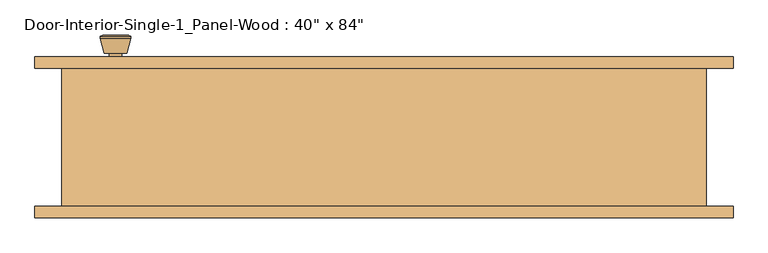
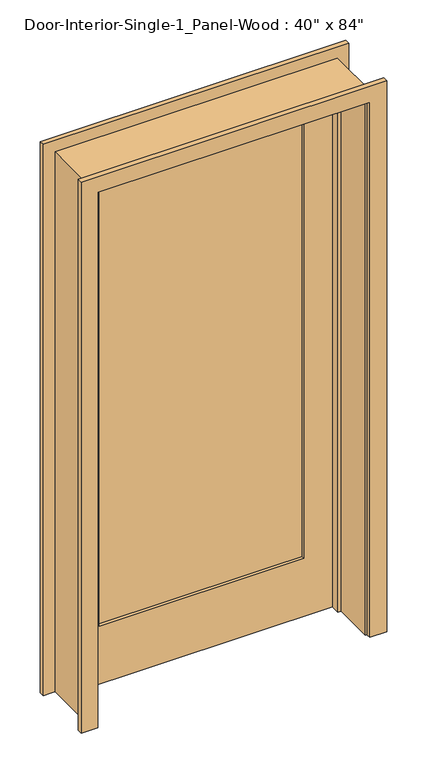
"""IFC4 building model written with IfcOpenShell, lengths in millimetres: door geometry."""

from ifc_helpers import new_model, si_unit, point, frame, frame_2d, origin, place, context, project, spatial, polyline, circle_curve, trimmed, segment, composite_curve, outline, extrude, faceted_brep, source, transform, mapped, element, save
from ifc_brep_helpers import plane_surface, cylinder_surface, revolved_surface, advanced_brep


def door_3a9a63a9(model_context):
    return source(origin(), model_context, "Body", "SolidModel", [
        advanced_brep(
        [(-444.5, 70.2, 914.4), (-434.5, 70.2, 914.4), (-454.5, 70.2, 914.4), (-424.0241324, 21.2, 914.4), (-444.5, 21.2, 914.4), (-464.9758676, 21.2, 914.4), (-419.5, 23.0278681, 914.4), (-469.5, 23.0278681, 914.4), (-419.5, 26.4915463, 914.4), (-469.5, 26.4915463, 914.4), (-425.863764, 51.2, 914.4), (-463.136236, 51.2, 914.4), (-434.5, 51.2, 914.4), (-454.5, 51.2, 914.4)],
        [
            (0, 1),
            (1, 2, circle_curve(frame((-444.5, 70.2, 914.4), z_axis=(0.0, 1.0, 0.0), x_axis=(-1.0, 0.0, 0.0)), 10.0)),
            (2, 0),
            (2, 1, circle_curve(frame((-444.5, 70.2, 914.4), z_axis=(0.0, 1.0, 0.0), x_axis=(-1.0, 0.0, 0.0)), 10.0)),
            (3, 4),
            (4, 5),
            (5, 3, circle_curve(frame((-444.5, 21.2, 914.4), z_axis=(0.0, -1.0, 0.0), x_axis=(-1.0, 0.0, 0.0)), 20.4758676)),
            (3, 5, circle_curve(frame((-444.5, 21.2, 914.4), z_axis=(0.0, -1.0, 0.0), x_axis=(-1.0, 0.0, 0.0)), 20.4758676)),
            (6, 3),
            (5, 7),
            (7, 6, circle_curve(frame((-444.5, 23.0278681, 914.4), z_axis=(0.0, -1.0, 0.0), x_axis=(-1.0, 0.0, 0.0)), 25.0)),
            (6, 7, circle_curve(frame((-444.5, 23.0278681, 914.4), z_axis=(0.0, -1.0, 0.0), x_axis=(-1.0, 0.0, 0.0)), 25.0)),
            (8, 6),
            (7, 9),
            (9, 8, circle_curve(frame((-444.5, 26.4915463, 914.4), z_axis=(0.0, -1.0, 0.0), x_axis=(-1.0, 0.0, 0.0)), 25.0)),
            (8, 9, circle_curve(frame((-444.5, 26.4915463, 914.4), z_axis=(0.0, -1.0, 0.0), x_axis=(-1.0, 0.0, 0.0)), 25.0)),
            (10, 8),
            (9, 11),
            (11, 10, circle_curve(frame((-444.5, 51.2, 914.4), z_axis=(0.0, -1.0, 0.0), x_axis=(-1.0, 0.0, 0.0)), 18.636236)),
            (10, 11, circle_curve(frame((-444.5, 51.2, 914.4), z_axis=(0.0, -1.0, 0.0), x_axis=(-1.0, 0.0, 0.0)), 18.636236)),
            (12, 10),
            (11, 13),
            (13, 12, circle_curve(frame((-444.5, 51.2, 914.4), z_axis=(0.0, -1.0, 0.0), x_axis=(-1.0, 0.0, 0.0)), 10.0)),
            (12, 13, circle_curve(frame((-444.5, 51.2, 914.4), z_axis=(0.0, -1.0, 0.0), x_axis=(-1.0, 0.0, 0.0)), 10.0)),
            (1, 12),
            (13, 2),
        ],
        [
            plane_surface(frame((-444.5, 70.2, 914.4), z_axis=(0.0, 1.0, 0.0), x_axis=(-1.0, 0.0, 0.0))),
            plane_surface(frame((-444.5, 21.2, 914.4), z_axis=(0.0, -1.0, 0.0), x_axis=(-1.0, 0.0, 0.0))),
            revolved_surface(polyline([(-464.9758676, 21.2, 914.4), (-469.5, 23.0278681, 914.4)]), (-444.5, 70.2, 914.4), (0.0, 1.0, 0.0)),
            cylinder_surface(frame((-444.5, 70.2, 914.4), z_axis=(0.0, 1.0, 0.0), x_axis=(-1.0, 0.0, 0.0)), 25.0),
            revolved_surface(polyline([(-469.5, 26.4915463, 914.4), (-463.136236, 51.2, 914.4)]), (-444.5, 70.2, 914.4), (0.0, 1.0, 0.0)),
            plane_surface(frame((-444.5, 51.2, 914.4), z_axis=(0.0, 1.0, 0.0), x_axis=(-1.0, 0.0, 0.0))),
            cylinder_surface(frame((-444.5, 70.2, 914.4), z_axis=(0.0, 1.0, 0.0), x_axis=(-1.0, 0.0, 0.0)), 10.0),
        ],
        [
            (0, [[1, 2, 3]]),
            (0, [[-3, 4, -1]]),
            (1, [[5, 6, 7]]),
            (1, [[-6, -5, 8]]),
            (2, [[9, -7, 10, 11]]),
            (2, [[-10, -8, -9, 12]]),
            (3, [[13, -11, 14, 15]]),
            (3, [[-14, -12, -13, 16]]),
            (4, [[17, -15, 18, 19]]),
            (4, [[-18, -16, -17, 20]]),
            (5, [[21, -19, 22, 23]]),
            (5, [[-22, -20, -21, 24]]),
            (6, [[25, -23, 26, -2]]),
            (6, [[-26, -24, -25, -4]]),
        ],
    ),
        extrude(outline(composite_curve([segment(trimmed(circle_curve(frame_2d((914.4, -444.5)), 30.0), [point((914.4, -474.5))], [point((914.4, -414.5))], False, "CARTESIAN"), True, "CONTINUOUS"), segment(trimmed(circle_curve(frame_2d((914.4, -444.5)), 30.0), [point((914.4, -414.5))], [point((914.4, -474.5))], False, "CARTESIAN"), True, "CONTINUOUS")], self_intersect=False)), frame((0.0, 70.2, 0.0), z_axis=(0.0, 1.0, 0.0), x_axis=(0.0, 0.0, 1.0)), (0.0, 0.0, 1.0), 6.0),
        advanced_brep(
        [(-444.5, 117.125, 914.4), (-454.5, 117.125, 914.4), (-434.5, 117.125, 914.4), (-424.0241324, 166.125, 914.4), (-464.9758676, 166.125, 914.4), (-444.5, 166.125, 914.4), (-419.5, 164.2971319, 914.4), (-469.5, 164.2971319, 914.4), (-419.5, 160.8334537, 914.4), (-469.5, 160.8334537, 914.4), (-425.863764, 136.125, 914.4), (-463.136236, 136.125, 914.4), (-434.5, 136.125, 914.4), (-454.5, 136.125, 914.4)],
        [
            (0, 1),
            (1, 2, circle_curve(frame((-444.5, 117.125, 914.4), z_axis=(0.0, -1.0, 0.0), x_axis=(-1.0, 0.0, 0.0)), 10.0)),
            (2, 0),
            (2, 1, circle_curve(frame((-444.5, 117.125, 914.4), z_axis=(0.0, -1.0, 0.0), x_axis=(-1.0, 0.0, 0.0)), 10.0)),
            (3, 4, circle_curve(frame((-444.5, 166.125, 914.4), z_axis=(0.0, 1.0, 0.0), x_axis=(-1.0, 0.0, 0.0)), 20.4758676)),
            (4, 5),
            (5, 3),
            (4, 3, circle_curve(frame((-444.5, 166.125, 914.4), z_axis=(0.0, 1.0, 0.0), x_axis=(-1.0, 0.0, 0.0)), 20.4758676)),
            (6, 7, circle_curve(frame((-444.5, 164.2971319, 914.4), z_axis=(0.0, 1.0, 0.0), x_axis=(-1.0, 0.0, 0.0)), 25.0)),
            (7, 4),
            (3, 6),
            (7, 6, circle_curve(frame((-444.5, 164.2971319, 914.4), z_axis=(0.0, 1.0, 0.0), x_axis=(-1.0, 0.0, 0.0)), 25.0)),
            (8, 9, circle_curve(frame((-444.5, 160.8334537, 914.4), z_axis=(0.0, 1.0, 0.0), x_axis=(-1.0, 0.0, 0.0)), 25.0)),
            (9, 7),
            (6, 8),
            (9, 8, circle_curve(frame((-444.5, 160.8334537, 914.4), z_axis=(0.0, 1.0, 0.0), x_axis=(-1.0, 0.0, 0.0)), 25.0)),
            (10, 11, circle_curve(frame((-444.5, 136.125, 914.4), z_axis=(0.0, 1.0, 0.0), x_axis=(-1.0, 0.0, 0.0)), 18.636236)),
            (11, 9),
            (8, 10),
            (11, 10, circle_curve(frame((-444.5, 136.125, 914.4), z_axis=(0.0, 1.0, 0.0), x_axis=(-1.0, 0.0, 0.0)), 18.636236)),
            (12, 13, circle_curve(frame((-444.5, 136.125, 914.4), z_axis=(0.0, 1.0, 0.0), x_axis=(-1.0, 0.0, 0.0)), 10.0)),
            (13, 11),
            (10, 12),
            (13, 12, circle_curve(frame((-444.5, 136.125, 914.4), z_axis=(0.0, 1.0, 0.0), x_axis=(-1.0, 0.0, 0.0)), 10.0)),
            (1, 13),
            (12, 2),
        ],
        [
            plane_surface(frame((-444.5, 117.125, 914.4), z_axis=(0.0, -1.0, 0.0), x_axis=(-1.0, 0.0, 0.0))),
            plane_surface(frame((-444.5, 166.125, 914.4), z_axis=(0.0, 1.0, 0.0), x_axis=(-1.0, 0.0, 0.0))),
            revolved_surface(polyline([(-464.9758676, 166.125, 914.4), (-469.5, 164.2971319, 914.4)]), (-444.5, 117.125, 914.4), (0.0, -1.0, 0.0)),
            cylinder_surface(frame((-444.5, 117.125, 914.4), z_axis=(0.0, -1.0, 0.0), x_axis=(-1.0, 0.0, 0.0)), 25.0),
            revolved_surface(polyline([(-469.5, 160.8334537, 914.4), (-463.136236, 136.125, 914.4)]), (-444.5, 117.125, 914.4), (0.0, -1.0, 0.0)),
            plane_surface(frame((-444.5, 136.125, 914.4), z_axis=(0.0, -1.0, 0.0), x_axis=(-1.0, 0.0, 0.0))),
            cylinder_surface(frame((-444.5, 117.125, 914.4), z_axis=(0.0, -1.0, 0.0), x_axis=(-1.0, 0.0, 0.0)), 10.0),
        ],
        [
            (0, [[1, 2, 3]]),
            (0, [[-3, 4, -1]]),
            (1, [[5, 6, 7]]),
            (1, [[8, -7, -6]]),
            (2, [[9, 10, -5, 11]]),
            (2, [[12, -11, -8, -10]]),
            (3, [[13, 14, -9, 15]]),
            (3, [[16, -15, -12, -14]]),
            (4, [[17, 18, -13, 19]]),
            (4, [[20, -19, -16, -18]]),
            (5, [[21, 22, -17, 23]]),
            (5, [[24, -23, -20, -22]]),
            (6, [[-2, 25, -21, 26]]),
            (6, [[-4, -26, -24, -25]]),
        ],
    ),
        extrude(outline(composite_curve([segment(trimmed(circle_curve(frame_2d((914.4, -444.5)), 30.0), [point((914.4, -474.5))], [point((914.4, -414.5))], False, "CARTESIAN"), True, "CONTINUOUS"), segment(trimmed(circle_curve(frame_2d((914.4, -444.5)), 30.0), [point((914.4, -414.5))], [point((914.4, -474.5))], False, "CARTESIAN"), True, "CONTINUOUS")], self_intersect=False)), frame((0.0, 111.125, 0.0), z_axis=(0.0, 1.0, 0.0), x_axis=(0.0, 0.0, 1.0)), (0.0, 0.0, 1.0), 6.0),
        faceted_brep([(533.4, 111.125, 0.0), (533.4, -117.475, 0.0), (508.0, -117.475, 0.0), (508.0, 41.275, 0.0), (495.3, 41.275, 0.0), (495.3, 76.2, 0.0), (508.0, 76.2, 0.0), (508.0, 111.125, 0.0), (533.4, 111.125, 2159.0), (533.4, -117.475, 2159.0), (-533.4, -117.475, 2159.0), (-533.4, -117.475, 0.0), (-508.0, -117.475, 0.0), (-508.0, -117.475, 2133.6), (508.0, -117.475, 2133.6), (508.0, 41.275, 2133.6), (-508.0, 41.275, 2133.6), (-508.0, 41.275, 0.0), (-495.3, 41.275, 0.0), (-495.3, 41.275, 2120.9), (495.3, 41.275, 2120.9), (495.3, 76.2, 2120.9), (-495.3, 76.2, 2120.9), (-495.3, 76.2, 0.0), (-508.0, 76.2, 0.0), (-508.0, 76.2, 2133.6), (508.0, 76.2, 2133.6), (508.0, 111.125, 2133.6), (-508.0, 111.125, 2133.6), (-508.0, 111.125, 0.0), (-533.4, 111.125, 0.0), (-533.4, 111.125, 2159.0)], [[[0, 1, 2, 3, 4, 5, 6, 7]], [[1, 0, 8, 9]], [[2, 1, 9, 10, 11, 12, 13, 14]], [[3, 2, 14, 15]], [[4, 3, 15, 16, 17, 18, 19, 20]], [[5, 4, 20, 21]], [[6, 5, 21, 22, 23, 24, 25, 26]], [[7, 6, 26, 27]], [[0, 7, 27, 28, 29, 30, 31, 8]], [[9, 8, 31, 10]], [[15, 14, 13, 16]], [[21, 20, 19, 22]], [[27, 26, 25, 28]], [[30, 29, 24, 23, 18, 17, 12, 11]], [[10, 31, 30, 11]], [[16, 13, 12, 17]], [[22, 19, 18, 23]], [[28, 25, 24, 29]]]),
        extrude(outline(polyline([(2133.6, -508.0), (0.0, -508.0), (0.0, 508.0), (2133.6, 508.0), (2133.6, -508.0)]), holes=[polyline([(2014.5375, -387.35), (2014.5375, 387.35), (231.775, 387.35), (231.775, -387.35), (2014.5375, -387.35)])]), frame((0.0, 76.2, 0.0), z_axis=(0.0, 1.0, 0.0), x_axis=(0.0, 0.0, 1.0)), (0.0, 0.0, 1.0), 34.925),
        extrude(outline(polyline([(387.35, 87.8416667), (-387.35, 87.8416667), (-387.35, 99.4833333), (387.35, 99.4833333), (387.35, 87.8416667)])), frame((0.0, 0.0, 231.775), z_axis=(0.0, 0.0, 1.0), x_axis=(1.0, 0.0, 0.0)), (0.0, 0.0, 1.0), 1782.7625),
        extrude(outline(polyline([(0.0, 514.35), (0.0, 577.85), (2203.45, 577.85), (2203.45, -577.85), (0.0, -577.85), (0.0, -514.35), (2139.95, -514.35), (2139.95, 514.35), (0.0, 514.35)])), frame((0.0, 111.125, 0.0), z_axis=(0.0, 1.0, 0.0), x_axis=(0.0, 0.0, 1.0)), (0.0, 0.0, 1.0), 19.05),
        extrude(outline(polyline([(0.0, 514.35), (0.0, 577.85), (2203.45, 577.85), (2203.45, -577.85), (0.0, -577.85), (0.0, -514.35), (2139.95, -514.35), (2139.95, 514.35), (0.0, 514.35)])), frame((0.0, -136.525, 0.0), z_axis=(0.0, 1.0, 0.0), x_axis=(0.0, 0.0, 1.0)), (0.0, 0.0, 1.0), 19.05),
    ])


if __name__ == "__main__":
    model = new_model("IFC4")
    model_context = context("Model", 3, world=origin())
    ifc_project = project(units=[si_unit("LENGTHUNIT", "METRE", prefix="MILLI")], contexts=[model_context])
    site = spatial("IfcSite", under=ifc_project)
    building = spatial("IfcBuilding", under=site)
    placement = place(None, origin())
    door_shape = door_3a9a63a9(model_context)
    element("IfcDoor", 1, ObjectType="Door-Interior-Single-1_Panel-Wood : 40\" x 84\"", at=placement, inside=building, context=model_context, shape_type="MappedRepresentation", body=[
        mapped(door_shape, transform((0.0, 0.0, 0.0), x_axis=(1.0, 0.0, 0.0), y_axis=(0.0, 1.0, 0.0), z_axis=(0.0, 0.0, 1.0))),
    ])
    save(model, "model.ifc")

# Revit data of these elements
# Type "Door-Interior-Single-1_Panel-Wood : 40\" x 84\""
#   Type Mark = "9"
#   Assembly Code = "C1020300"
#   Analytic Construction = "Wooden"
#   Top Rail = 0' - 4 11/16"
#   Thickness = 0' - 1 3/8"
#   Thermal Resistance (R) = 2.5876 (h·ft²·°F)/BTU
#   Swing Angle [instance default] = 90.00°
#   Stiles = 0' - 4 3/4"
#   Rough Width = 3' - 6"
#   Rough Height = 7' - 1"
#   Height = 7' - 0"
#   Width = 3' - 4"
#   Heat Transfer Coefficient (U) = 0.3865 BTU/(h·ft²·°F)
#   Bottom Rail = 0' - 9 1/8"
#   Trim Material = Cherry
#   Panel Material = door
#   Frame Material = Cherry
#   Door Handle Material = Aluminum
#   Visual Light Transmittance = 0
#   Solar Heat Gain Coefficient = 0
#   Wall Closure = (empty or 0)
#   Function = (empty or 0)
# Element 1 (IfcDoor, "Door-Interior-Single-1_Panel-Wood : 40\" x 84\"")
#   Materials on its faces: "Cherry", "Aluminum", "door"
# Materials
#   "Cherry": class "Wood", colour RGB 226 177 128, transparency 0, Description = "Prunus Serotina", Cost = 0
#   "door": class "Generic", colour RGB 120 120 120, transparency 0, Cost = 0
#   "Aluminum": class "Metal", colour RGB 247 247 247, transparency 0, Description = "Aluminum 6061", Cost = 0
